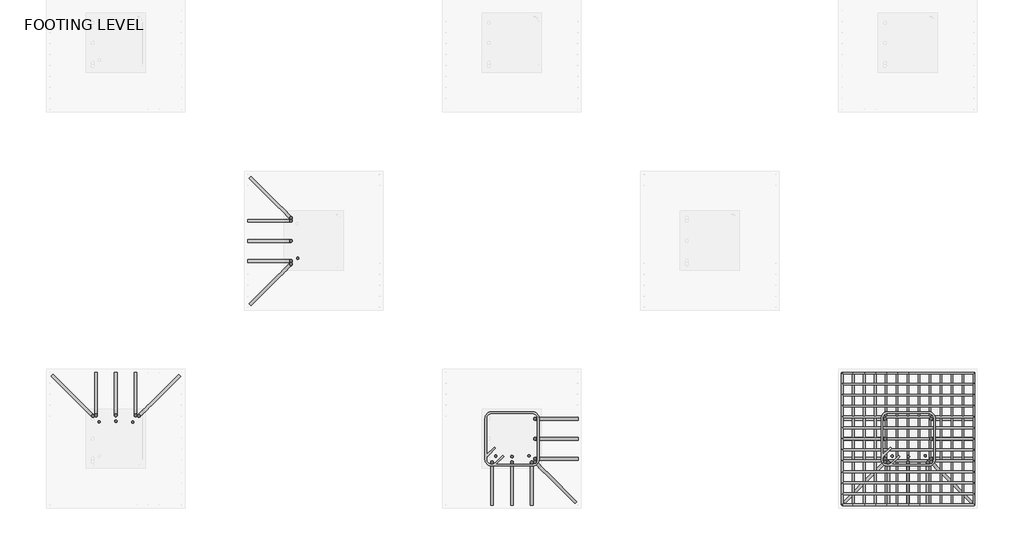
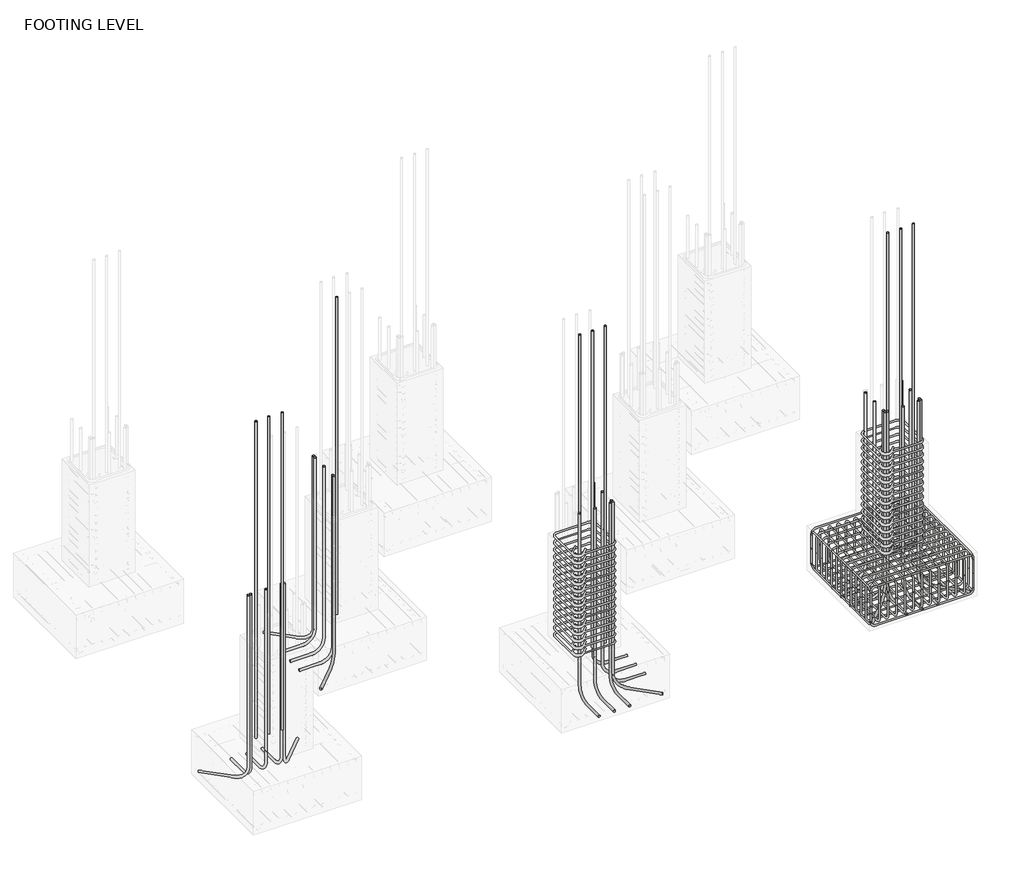
# One storey, part 3 of 10: 32 reinforcing bars.
"""IFC4 building model written with IfcOpenShell, lengths in millimetres."""

from ifc_helpers import new_model, si_unit, point, frame, origin, place, context, project, spatial, polyline, circle_curve, trimmed, segment, composite_curve, source, transform, mapped, element, save
from ifc_brep_helpers import swept_disk

model = new_model("IFC4")

# Units and contexts
model_context = context("Model", 3, world=origin())
ifc_project = project(units=[si_unit("LENGTHUNIT", "METRE", prefix="MILLI")], contexts=[model_context])

# Site, building, storey
site = spatial("IfcSite", under=ifc_project)
building = spatial("IfcBuilding", under=site)
storey = spatial("IfcBuildingStorey", under=building, Name="FOOTING LEVEL", Elevation=-2133.6)

# Reinforcing bars
placement = place(None, origin())
reinforcing_bar_shape = source(origin(), model_context, "Body", "SolidModel", [
    swept_disk(composite_curve([segment(polyline([(365.0730963, 756.4829396, -2583.0), (365.0730963, 756.4829396, -2905.1)]), True, "CONTINUOUS"), segment(trimmed(circle_curve(frame((274.8730963, 756.4829396, -2905.1), z_axis=(0.0, 1.0, 0.0), x_axis=(90.19999999999999, 0.0, 0.0)), 90.2), [point((365.0730963, 756.4829396, -2905.1))], [point((274.8730963, 756.4829396, -2995.3))], True, "CARTESIAN"), True, "CONTINUOUS"), segment(polyline([(274.8730963, 756.4829396, -2995.3), (-1572.9269037, 756.4829396, -2995.3)]), True, "CONTINUOUS"), segment(trimmed(circle_curve(frame((-1572.9269037, 756.4829396, -2905.1), z_axis=(0.0, 1.0, 0.0), x_axis=(0.0, 0.0, -90.20000000000027)), 90.2), [point((-1572.9269037, 756.4829396, -2995.3))], [point((-1663.1269037, 756.4829396, -2905.1))], True, "CARTESIAN"), True, "CONTINUOUS"), segment(polyline([(-1663.1269037, 756.4829396, -2905.1), (-1663.1269037, 756.4829396, -2583.0)]), True, "CONTINUOUS")], self_intersect=False), 12.7),
])
element("IfcReinforcingBar", 1, at=placement, inside=storey, context=model_context, shape_type="MappedRepresentation", body=[
    mapped(reinforcing_bar_shape, transform((0.0, 0.0, 0.0), x_axis=(1.0, 0.0, 0.0), y_axis=(0.0, 1.0, 0.0), z_axis=(0.0, 0.0, 1.0))),
    mapped(reinforcing_bar_shape, transform((0.0, -169.0166667, 0.0), x_axis=(1.0, 0.0, 0.0), y_axis=(0.0, 1.0, 0.0), z_axis=(0.0, 0.0, 1.0))),
    mapped(reinforcing_bar_shape, transform((0.0, -338.0333333, 0.0), x_axis=(1.0, 0.0, 0.0), y_axis=(0.0, 1.0, 0.0), z_axis=(0.0, 0.0, 1.0))),
    mapped(reinforcing_bar_shape, transform((0.0, -507.05, 0.0), x_axis=(1.0, 0.0, 0.0), y_axis=(0.0, 1.0, 0.0), z_axis=(0.0, 0.0, 1.0))),
    mapped(reinforcing_bar_shape, transform((0.0, -676.0666667, 0.0), x_axis=(1.0, 0.0, 0.0), y_axis=(0.0, 1.0, 0.0), z_axis=(0.0, 0.0, 1.0))),
    mapped(reinforcing_bar_shape, transform((0.0, -845.0833333, 0.0), x_axis=(1.0, 0.0, 0.0), y_axis=(0.0, 1.0, 0.0), z_axis=(0.0, 0.0, 1.0))),
    mapped(reinforcing_bar_shape, transform((0.0, -1014.1, 0.0), x_axis=(1.0, 0.0, 0.0), y_axis=(0.0, 1.0, 0.0), z_axis=(0.0, 0.0, 1.0))),
    mapped(reinforcing_bar_shape, transform((0.0, -1183.1166667, 0.0), x_axis=(1.0, 0.0, 0.0), y_axis=(0.0, 1.0, 0.0), z_axis=(0.0, 0.0, 1.0))),
    mapped(reinforcing_bar_shape, transform((0.0, -1352.1333333, 0.0), x_axis=(1.0, 0.0, 0.0), y_axis=(0.0, 1.0, 0.0), z_axis=(0.0, 0.0, 1.0))),
    mapped(reinforcing_bar_shape, transform((0.0, -1521.15, 0.0), x_axis=(1.0, 0.0, 0.0), y_axis=(0.0, 1.0, 0.0), z_axis=(0.0, 0.0, 1.0))),
    mapped(reinforcing_bar_shape, transform((0.0, -1690.1666667, 0.0), x_axis=(1.0, 0.0, 0.0), y_axis=(0.0, 1.0, 0.0), z_axis=(0.0, 0.0, 1.0))),
    mapped(reinforcing_bar_shape, transform((0.0, -1859.1833333, 0.0), x_axis=(1.0, 0.0, 0.0), y_axis=(0.0, 1.0, 0.0), z_axis=(0.0, 0.0, 1.0))),
    mapped(reinforcing_bar_shape, transform((0.0, -2028.2, 0.0), x_axis=(1.0, 0.0, 0.0), y_axis=(0.0, 1.0, 0.0), z_axis=(0.0, 0.0, 1.0))),
])
reinforcing_bar_2_shape = source(origin(), model_context, "Body", "SolidModel", [
    swept_disk(composite_curve([segment(polyline([(-1663.1269037, 756.4829396, -2598.6), (-1663.1269037, 756.4829396, -2276.5)]), True, "CONTINUOUS"), segment(trimmed(circle_curve(frame((-1572.9269037, 756.4829396, -2276.5), z_axis=(0.0, 1.0, 0.0), x_axis=(-90.20000000000005, 0.0, 0.0)), 90.2), [point((-1663.1269037, 756.4829396, -2276.5))], [point((-1572.9269037, 756.4829396, -2186.3))], True, "CARTESIAN"), True, "CONTINUOUS"), segment(polyline([(-1572.9269037, 756.4829396, -2186.3), (274.8730963, 756.4829396, -2186.3)]), True, "CONTINUOUS"), segment(trimmed(circle_curve(frame((274.8730963, 756.4829396, -2276.5), z_axis=(0.0, 1.0, 0.0), x_axis=(0.0, 0.0, 90.19999999999982)), 90.2), [point((274.8730963, 756.4829396, -2186.3))], [point((365.0730963, 756.4829396, -2276.5))], True, "CARTESIAN"), True, "CONTINUOUS"), segment(polyline([(365.0730963, 756.4829396, -2276.5), (365.0730963, 756.4829396, -2598.6)]), True, "CONTINUOUS")], self_intersect=False), 12.7),
])
element("IfcReinforcingBar", 2, at=placement, inside=storey, context=model_context, shape_type="MappedRepresentation", body=[
    mapped(reinforcing_bar_2_shape, transform((0.0, 0.0, 0.0), x_axis=(1.0, 0.0, 0.0), y_axis=(0.0, 1.0, 0.0), z_axis=(0.0, 0.0, 1.0))),
    mapped(reinforcing_bar_2_shape, transform((0.0, -169.0166667, 0.0), x_axis=(1.0, 0.0, 0.0), y_axis=(0.0, 1.0, 0.0), z_axis=(0.0, 0.0, 1.0))),
    mapped(reinforcing_bar_2_shape, transform((0.0, -338.0333333, 0.0), x_axis=(1.0, 0.0, 0.0), y_axis=(0.0, 1.0, 0.0), z_axis=(0.0, 0.0, 1.0))),
    mapped(reinforcing_bar_2_shape, transform((0.0, -507.05, 0.0), x_axis=(1.0, 0.0, 0.0), y_axis=(0.0, 1.0, 0.0), z_axis=(0.0, 0.0, 1.0))),
    mapped(reinforcing_bar_2_shape, transform((0.0, -676.0666667, 0.0), x_axis=(1.0, 0.0, 0.0), y_axis=(0.0, 1.0, 0.0), z_axis=(0.0, 0.0, 1.0))),
    mapped(reinforcing_bar_2_shape, transform((0.0, -845.0833333, 0.0), x_axis=(1.0, 0.0, 0.0), y_axis=(0.0, 1.0, 0.0), z_axis=(0.0, 0.0, 1.0))),
    mapped(reinforcing_bar_2_shape, transform((0.0, -1014.1, 0.0), x_axis=(1.0, 0.0, 0.0), y_axis=(0.0, 1.0, 0.0), z_axis=(0.0, 0.0, 1.0))),
    mapped(reinforcing_bar_2_shape, transform((0.0, -1183.1166667, 0.0), x_axis=(1.0, 0.0, 0.0), y_axis=(0.0, 1.0, 0.0), z_axis=(0.0, 0.0, 1.0))),
    mapped(reinforcing_bar_2_shape, transform((0.0, -1352.1333333, 0.0), x_axis=(1.0, 0.0, 0.0), y_axis=(0.0, 1.0, 0.0), z_axis=(0.0, 0.0, 1.0))),
    mapped(reinforcing_bar_2_shape, transform((0.0, -1521.15, 0.0), x_axis=(1.0, 0.0, 0.0), y_axis=(0.0, 1.0, 0.0), z_axis=(0.0, 0.0, 1.0))),
    mapped(reinforcing_bar_2_shape, transform((0.0, -1690.1666667, 0.0), x_axis=(1.0, 0.0, 0.0), y_axis=(0.0, 1.0, 0.0), z_axis=(0.0, 0.0, 1.0))),
    mapped(reinforcing_bar_2_shape, transform((0.0, -1859.1833333, 0.0), x_axis=(1.0, 0.0, 0.0), y_axis=(0.0, 1.0, 0.0), z_axis=(0.0, 0.0, 1.0))),
    mapped(reinforcing_bar_2_shape, transform((0.0, -2028.2, 0.0), x_axis=(1.0, 0.0, 0.0), y_axis=(0.0, 1.0, 0.0), z_axis=(0.0, 0.0, 1.0))),
])
reinforcing_bar_3_shape = source(origin(), model_context, "Body", "SolidModel", [
    swept_disk(composite_curve([segment(polyline([(365.0730963, -1271.7170604, -2559.4978077), (365.0730963, -1271.7170604, -2881.5978077)]), True, "CONTINUOUS"), segment(trimmed(circle_curve(frame((365.0730963, -1181.5170604, -2881.5978077), z_axis=(1.0, 0.0, 0.0), x_axis=(0.0, -90.20000000000005, 0.0)), 90.2), [point((365.0730963, -1271.7170604, -2881.5978077))], [point((365.0730963, -1181.5170604, -2971.7978077))], True, "CARTESIAN"), True, "CONTINUOUS"), segment(polyline([(365.0730963, -1181.5170604, -2971.7978077), (365.0730963, 666.2829396, -2971.7978077)]), True, "CONTINUOUS"), segment(trimmed(circle_curve(frame((365.0730963, 666.2829396, -2881.5978077), z_axis=(1.0, 0.0, 0.0), x_axis=(0.0, 0.0, -90.19999999999982)), 90.2), [point((365.0730963, 666.2829396, -2971.7978077))], [point((365.0730963, 756.4829396, -2881.5978077))], True, "CARTESIAN"), True, "CONTINUOUS"), segment(polyline([(365.0730963, 756.4829396, -2881.5978077), (365.0730963, 756.4829396, -2559.4978077)]), True, "CONTINUOUS")], self_intersect=False), 12.7),
])
element("IfcReinforcingBar", 3, at=placement, inside=storey, context=model_context, shape_type="MappedRepresentation", body=[
    mapped(reinforcing_bar_3_shape, transform((0.0, 0.0, 0.0), x_axis=(1.0, 0.0, 0.0), y_axis=(0.0, 1.0, 0.0), z_axis=(0.0, 0.0, 1.0))),
    mapped(reinforcing_bar_3_shape, transform((-169.0166667, 0.0, 0.0), x_axis=(1.0, 0.0, 0.0), y_axis=(0.0, 1.0, 0.0), z_axis=(0.0, 0.0, 1.0))),
    mapped(reinforcing_bar_3_shape, transform((-338.0333333, 0.0, 0.0), x_axis=(1.0, 0.0, 0.0), y_axis=(0.0, 1.0, 0.0), z_axis=(0.0, 0.0, 1.0))),
    mapped(reinforcing_bar_3_shape, transform((-507.05, 0.0, 0.0), x_axis=(1.0, 0.0, 0.0), y_axis=(0.0, 1.0, 0.0), z_axis=(0.0, 0.0, 1.0))),
    mapped(reinforcing_bar_3_shape, transform((-676.0666667, 0.0, 0.0), x_axis=(1.0, 0.0, 0.0), y_axis=(0.0, 1.0, 0.0), z_axis=(0.0, 0.0, 1.0))),
    mapped(reinforcing_bar_3_shape, transform((-845.0833333, 0.0, 0.0), x_axis=(1.0, 0.0, 0.0), y_axis=(0.0, 1.0, 0.0), z_axis=(0.0, 0.0, 1.0))),
    mapped(reinforcing_bar_3_shape, transform((-1014.1, 0.0, 0.0), x_axis=(1.0, 0.0, 0.0), y_axis=(0.0, 1.0, 0.0), z_axis=(0.0, 0.0, 1.0))),
    mapped(reinforcing_bar_3_shape, transform((-1183.1166667, 0.0, 0.0), x_axis=(1.0, 0.0, 0.0), y_axis=(0.0, 1.0, 0.0), z_axis=(0.0, 0.0, 1.0))),
    mapped(reinforcing_bar_3_shape, transform((-1352.1333333, 0.0, 0.0), x_axis=(1.0, 0.0, 0.0), y_axis=(0.0, 1.0, 0.0), z_axis=(0.0, 0.0, 1.0))),
    mapped(reinforcing_bar_3_shape, transform((-1521.15, 0.0, 0.0), x_axis=(1.0, 0.0, 0.0), y_axis=(0.0, 1.0, 0.0), z_axis=(0.0, 0.0, 1.0))),
    mapped(reinforcing_bar_3_shape, transform((-1690.1666667, 0.0, 0.0), x_axis=(1.0, 0.0, 0.0), y_axis=(0.0, 1.0, 0.0), z_axis=(0.0, 0.0, 1.0))),
    mapped(reinforcing_bar_3_shape, transform((-1859.1833333, 0.0, 0.0), x_axis=(1.0, 0.0, 0.0), y_axis=(0.0, 1.0, 0.0), z_axis=(0.0, 0.0, 1.0))),
    mapped(reinforcing_bar_3_shape, transform((-2028.2, 0.0, 0.0), x_axis=(1.0, 0.0, 0.0), y_axis=(0.0, 1.0, 0.0), z_axis=(0.0, 0.0, 1.0))),
])
reinforcing_bar_4_shape = source(origin(), model_context, "Body", "SolidModel", [
    swept_disk(composite_curve([segment(polyline([(-1663.1269037, -1271.7170604, -2622.9919875), (-1663.1269037, -1271.7170604, -2300.8919875)]), True, "CONTINUOUS"), segment(trimmed(circle_curve(frame((-1663.1269037, -1181.5170604, -2300.8919875), z_axis=(-1.0, 0.0, 0.0), x_axis=(0.0, -90.20000000000005, 0.0)), 90.2), [point((-1663.1269037, -1271.7170604, -2300.8919875))], [point((-1663.1269037, -1181.5170604, -2210.6919875))], True, "CARTESIAN"), True, "CONTINUOUS"), segment(polyline([(-1663.1269037, -1181.5170604, -2210.6919875), (-1663.1269037, 666.2829396, -2210.6919875)]), True, "CONTINUOUS"), segment(trimmed(circle_curve(frame((-1663.1269037, 666.2829396, -2300.8919875), z_axis=(-1.0, 0.0, 0.0), x_axis=(0.0, 0.0, 90.20000000000027)), 90.2), [point((-1663.1269037, 666.2829396, -2210.6919875))], [point((-1663.1269037, 756.4829396, -2300.8919875))], True, "CARTESIAN"), True, "CONTINUOUS"), segment(polyline([(-1663.1269037, 756.4829396, -2300.8919875), (-1663.1269037, 756.4829396, -2622.9919875)]), True, "CONTINUOUS")], self_intersect=False), 12.7),
])
element("IfcReinforcingBar", 4, at=placement, inside=storey, context=model_context, shape_type="MappedRepresentation", body=[
    mapped(reinforcing_bar_4_shape, transform((0.0, 0.0, 0.0), x_axis=(1.0, 0.0, 0.0), y_axis=(0.0, 1.0, 0.0), z_axis=(0.0, 0.0, 1.0))),
    mapped(reinforcing_bar_4_shape, transform((169.0166667, 0.0, 0.0), x_axis=(1.0, 0.0, 0.0), y_axis=(0.0, 1.0, 0.0), z_axis=(0.0, 0.0, 1.0))),
    mapped(reinforcing_bar_4_shape, transform((338.0333333, 0.0, 0.0), x_axis=(1.0, 0.0, 0.0), y_axis=(0.0, 1.0, 0.0), z_axis=(0.0, 0.0, 1.0))),
    mapped(reinforcing_bar_4_shape, transform((507.05, 0.0, 0.0), x_axis=(1.0, 0.0, 0.0), y_axis=(0.0, 1.0, 0.0), z_axis=(0.0, 0.0, 1.0))),
    mapped(reinforcing_bar_4_shape, transform((676.0666667, 0.0, 0.0), x_axis=(1.0, 0.0, 0.0), y_axis=(0.0, 1.0, 0.0), z_axis=(0.0, 0.0, 1.0))),
    mapped(reinforcing_bar_4_shape, transform((845.0833333, 0.0, 0.0), x_axis=(1.0, 0.0, 0.0), y_axis=(0.0, 1.0, 0.0), z_axis=(0.0, 0.0, 1.0))),
    mapped(reinforcing_bar_4_shape, transform((1014.1, 0.0, 0.0), x_axis=(1.0, 0.0, 0.0), y_axis=(0.0, 1.0, 0.0), z_axis=(0.0, 0.0, 1.0))),
    mapped(reinforcing_bar_4_shape, transform((1183.1166667, 0.0, 0.0), x_axis=(1.0, 0.0, 0.0), y_axis=(0.0, 1.0, 0.0), z_axis=(0.0, 0.0, 1.0))),
    mapped(reinforcing_bar_4_shape, transform((1352.1333333, 0.0, 0.0), x_axis=(1.0, 0.0, 0.0), y_axis=(0.0, 1.0, 0.0), z_axis=(0.0, 0.0, 1.0))),
    mapped(reinforcing_bar_4_shape, transform((1521.15, 0.0, 0.0), x_axis=(1.0, 0.0, 0.0), y_axis=(0.0, 1.0, 0.0), z_axis=(0.0, 0.0, 1.0))),
    mapped(reinforcing_bar_4_shape, transform((1690.1666667, 0.0, 0.0), x_axis=(1.0, 0.0, 0.0), y_axis=(0.0, 1.0, 0.0), z_axis=(0.0, 0.0, 1.0))),
    mapped(reinforcing_bar_4_shape, transform((1859.1833333, 0.0, 0.0), x_axis=(1.0, 0.0, 0.0), y_axis=(0.0, 1.0, 0.0), z_axis=(0.0, 0.0, 1.0))),
    mapped(reinforcing_bar_4_shape, transform((2028.2, 0.0, 0.0), x_axis=(1.0, 0.0, 0.0), y_axis=(0.0, 1.0, 0.0), z_axis=(0.0, 0.0, 1.0))),
])
reinforcing_bar_5_shape = source(origin(), model_context, "Body", "SolidModel", [
    swept_disk(composite_curve([segment(polyline([(-6882.1462687, -522.2984887, 0.0), (-6995.545872, -635.6980921, 0.0)]), True, "CONTINUOUS"), segment(trimmed(circle_curve(frame((-7059.3269037, -571.9170604, 0.0), z_axis=(0.0, 0.0, -1.0), x_axis=(63.78103170000031, -63.781031700000085, 0.0)), 90.2), [point((-6995.545872, -635.6980921, 0.0))], [point((-7149.5269037, -571.9170604, 0.0))], True, "CARTESIAN"), True, "CONTINUOUS"), segment(polyline([(-7149.5269037, -571.9170604, 0.0), (-7149.5269037, 56.6829396, 0.0)]), True, "CONTINUOUS"), segment(trimmed(circle_curve(frame((-7059.3269037, 56.6829396, 0.0), z_axis=(0.0, 0.0, -1.0), x_axis=(-90.19999999999982, 0.0, 0.0)), 90.2), [point((-7149.5269037, 56.6829396, 0.0))], [point((-7059.3269037, 146.8829396, 0.0))], True, "CARTESIAN"), True, "CONTINUOUS"), segment(polyline([(-7059.3269037, 146.8829396, 0.0), (-6430.7269037, 146.8829396, 0.0)]), True, "CONTINUOUS"), segment(trimmed(circle_curve(frame((-6430.7269037, 56.7273645, 2.8305953), z_axis=(0.0, -0.03138132276777647, -0.9995074850051623), x_axis=(0.0, 90.1555751, -2.8305953)), 90.2), [point((-6430.7269037, 146.8829396, 0.0))], [point((-6340.5269037, 56.7273645, 2.8305953))], True, "CARTESIAN"), True, "CONTINUOUS"), segment(polyline([(-6340.5269037, 56.7273645, 2.8305953), (-6340.5269037, -571.9614853, 22.5694047)]), True, "CONTINUOUS"), segment(trimmed(circle_curve(frame((-6430.7269037, -571.9614853, 22.5694047), z_axis=(0.0, -0.03138132276777647, -0.9995074850051623), x_axis=(90.19999999999982, 0.0, 0.0)), 90.2), [point((-6340.5269037, -571.9614853, 22.5694047))], [point((-6430.7269037, -662.1170604, 25.4))], True, "CARTESIAN"), True, "CONTINUOUS"), segment(polyline([(-6430.7269037, -662.1170604, 25.4), (-7059.3269037, -662.1170604, 25.4)]), True, "CONTINUOUS"), segment(trimmed(circle_curve(frame((-7059.3269037, -571.9170604, 25.4), z_axis=(0.0, 0.0, -1.0), x_axis=(0.0, -90.20000000000005, 0.0)), 90.2), [point((-7059.3269037, -662.1170604, 25.4))], [point((-7123.1079353, -508.1360287, 25.4))], True, "CARTESIAN"), True, "CONTINUOUS"), segment(polyline([(-7123.1079353, -508.1360287, 25.4), (-7009.708332, -394.7364254, 25.4)]), True, "CONTINUOUS")], self_intersect=False), 12.7),
])
element("IfcReinforcingBar", 5, at=placement, inside=storey, context=model_context, shape_type="MappedRepresentation", body=[
    mapped(reinforcing_bar_5_shape, transform((0.0, 0.0, 0.0), x_axis=(1.0, 0.0, 0.0), y_axis=(0.0, 1.0, 0.0), z_axis=(0.0, 0.0, 1.0))),
    mapped(reinforcing_bar_5_shape, transform((0.0, 0.0, -148.6357143), x_axis=(1.0, 0.0, 0.0), y_axis=(0.0, 1.0, 0.0), z_axis=(0.0, 0.0, 1.0))),
    mapped(reinforcing_bar_5_shape, transform((0.0, 0.0, -297.2714286), x_axis=(1.0, 0.0, 0.0), y_axis=(0.0, 1.0, 0.0), z_axis=(0.0, 0.0, 1.0))),
    mapped(reinforcing_bar_5_shape, transform((0.0, 0.0, -445.9071429), x_axis=(1.0, 0.0, 0.0), y_axis=(0.0, 1.0, 0.0), z_axis=(0.0, 0.0, 1.0))),
    mapped(reinforcing_bar_5_shape, transform((0.0, 0.0, -594.5428571), x_axis=(1.0, 0.0, 0.0), y_axis=(0.0, 1.0, 0.0), z_axis=(0.0, 0.0, 1.0))),
    mapped(reinforcing_bar_5_shape, transform((0.0, 0.0, -743.1785714), x_axis=(1.0, 0.0, 0.0), y_axis=(0.0, 1.0, 0.0), z_axis=(0.0, 0.0, 1.0))),
    mapped(reinforcing_bar_5_shape, transform((0.0, 0.0, -891.8142857), x_axis=(1.0, 0.0, 0.0), y_axis=(0.0, 1.0, 0.0), z_axis=(0.0, 0.0, 1.0))),
    mapped(reinforcing_bar_5_shape, transform((0.0, 0.0, -1040.45), x_axis=(1.0, 0.0, 0.0), y_axis=(0.0, 1.0, 0.0), z_axis=(0.0, 0.0, 1.0))),
    mapped(reinforcing_bar_5_shape, transform((0.0, 0.0, -1189.0857143), x_axis=(1.0, 0.0, 0.0), y_axis=(0.0, 1.0, 0.0), z_axis=(0.0, 0.0, 1.0))),
    mapped(reinforcing_bar_5_shape, transform((0.0, 0.0, -1337.7214286), x_axis=(1.0, 0.0, 0.0), y_axis=(0.0, 1.0, 0.0), z_axis=(0.0, 0.0, 1.0))),
    mapped(reinforcing_bar_5_shape, transform((0.0, 0.0, -1486.3571429), x_axis=(1.0, 0.0, 0.0), y_axis=(0.0, 1.0, 0.0), z_axis=(0.0, 0.0, 1.0))),
    mapped(reinforcing_bar_5_shape, transform((0.0, 0.0, -1634.9928571), x_axis=(1.0, 0.0, 0.0), y_axis=(0.0, 1.0, 0.0), z_axis=(0.0, 0.0, 1.0))),
    mapped(reinforcing_bar_5_shape, transform((0.0, 0.0, -1783.6285714), x_axis=(1.0, 0.0, 0.0), y_axis=(0.0, 1.0, 0.0), z_axis=(0.0, 0.0, 1.0))),
    mapped(reinforcing_bar_5_shape, transform((0.0, 0.0, -1932.2642857), x_axis=(1.0, 0.0, 0.0), y_axis=(0.0, 1.0, 0.0), z_axis=(0.0, 0.0, 1.0))),
    mapped(reinforcing_bar_5_shape, transform((0.0, 0.0, -2080.9), x_axis=(1.0, 0.0, 0.0), y_axis=(0.0, 1.0, 0.0), z_axis=(0.0, 0.0, 1.0))),
])
reinforcing_bar_6_shape = source(origin(), model_context, "Body", "SolidModel", [
    swept_disk(composite_curve([segment(polyline([(-786.1462687, -522.2984887, 0.0), (-899.545872, -635.6980921, 0.0)]), True, "CONTINUOUS"), segment(trimmed(circle_curve(frame((-963.3269037, -571.9170604, 0.0), z_axis=(0.0, 0.0, -1.0), x_axis=(63.78103169999997, -63.781031700000085, 0.0)), 90.2), [point((-899.545872, -635.6980921, 0.0))], [point((-1053.5269037, -571.9170604, 0.0))], True, "CARTESIAN"), True, "CONTINUOUS"), segment(polyline([(-1053.5269037, -571.9170604, 0.0), (-1053.5269037, 56.6829396, 0.0)]), True, "CONTINUOUS"), segment(trimmed(circle_curve(frame((-963.3269037, 56.6829396, 0.0), z_axis=(0.0, 0.0, -1.0), x_axis=(-90.20000000000005, 0.0, 0.0)), 90.2), [point((-1053.5269037, 56.6829396, 0.0))], [point((-963.3269037, 146.8829396, 0.0))], True, "CARTESIAN"), True, "CONTINUOUS"), segment(polyline([(-963.3269037, 146.8829396, 0.0), (-334.7269037, 146.8829396, 0.0)]), True, "CONTINUOUS"), segment(trimmed(circle_curve(frame((-334.7269037, 56.7273645, 2.8305953), z_axis=(0.0, -0.03138132276777647, -0.9995074850051623), x_axis=(0.0, 90.1555751, -2.8305953)), 90.2), [point((-334.7269037, 146.8829396, 0.0))], [point((-244.5269037, 56.7273645, 2.8305953))], True, "CARTESIAN"), True, "CONTINUOUS"), segment(polyline([(-244.5269037, 56.7273645, 2.8305953), (-244.5269037, -571.9614853, 22.5694047)]), True, "CONTINUOUS"), segment(trimmed(circle_curve(frame((-334.7269037, -571.9614853, 22.5694047), z_axis=(0.0, -0.03138132276777647, -0.9995074850051623), x_axis=(90.19999999999999, 0.0, 0.0)), 90.2), [point((-244.5269037, -571.9614853, 22.5694047))], [point((-334.7269037, -662.1170604, 25.4))], True, "CARTESIAN"), True, "CONTINUOUS"), segment(polyline([(-334.7269037, -662.1170604, 25.4), (-963.3269037, -662.1170604, 25.4)]), True, "CONTINUOUS"), segment(trimmed(circle_curve(frame((-963.3269037, -571.9170604, 25.4), z_axis=(0.0, 0.0, -1.0), x_axis=(0.0, -90.20000000000005, 0.0)), 90.2), [point((-963.3269037, -662.1170604, 25.4))], [point((-1027.1079353, -508.1360287, 25.4))], True, "CARTESIAN"), True, "CONTINUOUS"), segment(polyline([(-1027.1079353, -508.1360287, 25.4), (-913.708332, -394.7364254, 25.4)]), True, "CONTINUOUS")], self_intersect=False), 12.7),
])
element("IfcReinforcingBar", 6, at=placement, inside=storey, context=model_context, shape_type="MappedRepresentation", body=[
    mapped(reinforcing_bar_6_shape, transform((0.0, 0.0, 0.0), x_axis=(1.0, 0.0, 0.0), y_axis=(0.0, 1.0, 0.0), z_axis=(0.0, 0.0, 1.0))),
    mapped(reinforcing_bar_6_shape, transform((0.0, 0.0, -148.6357143), x_axis=(1.0, 0.0, 0.0), y_axis=(0.0, 1.0, 0.0), z_axis=(0.0, 0.0, 1.0))),
    mapped(reinforcing_bar_6_shape, transform((0.0, 0.0, -297.2714286), x_axis=(1.0, 0.0, 0.0), y_axis=(0.0, 1.0, 0.0), z_axis=(0.0, 0.0, 1.0))),
    mapped(reinforcing_bar_6_shape, transform((0.0, 0.0, -445.9071429), x_axis=(1.0, 0.0, 0.0), y_axis=(0.0, 1.0, 0.0), z_axis=(0.0, 0.0, 1.0))),
    mapped(reinforcing_bar_6_shape, transform((0.0, 0.0, -594.5428571), x_axis=(1.0, 0.0, 0.0), y_axis=(0.0, 1.0, 0.0), z_axis=(0.0, 0.0, 1.0))),
    mapped(reinforcing_bar_6_shape, transform((0.0, 0.0, -743.1785714), x_axis=(1.0, 0.0, 0.0), y_axis=(0.0, 1.0, 0.0), z_axis=(0.0, 0.0, 1.0))),
    mapped(reinforcing_bar_6_shape, transform((0.0, 0.0, -891.8142857), x_axis=(1.0, 0.0, 0.0), y_axis=(0.0, 1.0, 0.0), z_axis=(0.0, 0.0, 1.0))),
    mapped(reinforcing_bar_6_shape, transform((0.0, 0.0, -1040.45), x_axis=(1.0, 0.0, 0.0), y_axis=(0.0, 1.0, 0.0), z_axis=(0.0, 0.0, 1.0))),
    mapped(reinforcing_bar_6_shape, transform((0.0, 0.0, -1189.0857143), x_axis=(1.0, 0.0, 0.0), y_axis=(0.0, 1.0, 0.0), z_axis=(0.0, 0.0, 1.0))),
    mapped(reinforcing_bar_6_shape, transform((0.0, 0.0, -1337.7214286), x_axis=(1.0, 0.0, 0.0), y_axis=(0.0, 1.0, 0.0), z_axis=(0.0, 0.0, 1.0))),
    mapped(reinforcing_bar_6_shape, transform((0.0, 0.0, -1486.3571429), x_axis=(1.0, 0.0, 0.0), y_axis=(0.0, 1.0, 0.0), z_axis=(0.0, 0.0, 1.0))),
    mapped(reinforcing_bar_6_shape, transform((0.0, 0.0, -1634.9928571), x_axis=(1.0, 0.0, 0.0), y_axis=(0.0, 1.0, 0.0), z_axis=(0.0, 0.0, 1.0))),
    mapped(reinforcing_bar_6_shape, transform((0.0, 0.0, -1783.6285714), x_axis=(1.0, 0.0, 0.0), y_axis=(0.0, 1.0, 0.0), z_axis=(0.0, 0.0, 1.0))),
    mapped(reinforcing_bar_6_shape, transform((0.0, 0.0, -1932.2642857), x_axis=(1.0, 0.0, 0.0), y_axis=(0.0, 1.0, 0.0), z_axis=(0.0, 0.0, 1.0))),
    mapped(reinforcing_bar_6_shape, transform((0.0, 0.0, -2080.9), x_axis=(1.0, 0.0, 0.0), y_axis=(0.0, 1.0, 0.0), z_axis=(0.0, 0.0, 1.0))),
])
element("IfcReinforcingBar", 7, at=placement, inside=storey, context=model_context, shape_type="SolidModel", body=[
    swept_disk(composite_curve([segment(polyline([(331.4269893, -1238.0709533, -2976.5), (-115.5238015, -791.1201626, -2976.5)]), True, "CONTINUOUS"), segment(trimmed(circle_curve(frame((-115.5238015, -791.1201626, -2722.5), z_axis=(0.7071067811865508, 0.7071067811865444, 0.0), x_axis=(0.0, 0.0, -254.0)), 254.0), [point((-115.5238015, -791.1201626, -2976.5))], [point((-295.1289239, -611.5150401, -2722.5))], True, "CARTESIAN"), True, "CONTINUOUS"), segment(polyline([(-295.1289239, -611.5150401, -2722.5), (-295.1289239, -611.5150401, 874.4)]), True, "CONTINUOUS")], self_intersect=False), 21.5),
])
element("IfcReinforcingBar", 8, at=placement, inside=storey, context=model_context, shape_type="SolidModel", body=[
    swept_disk(composite_curve([segment(polyline([(-1629.4807966, -1238.0709533, -2976.5), (-1182.5300058, -791.1201626, -2976.5)]), True, "CONTINUOUS"), segment(trimmed(circle_curve(frame((-1182.5300058, -791.1201626, -2722.5), z_axis=(0.7071067811865475, -0.7071067811865477, 0.0), x_axis=(0.0, 0.0, -254.0)), 254.0), [point((-1182.5300058, -791.1201626, -2976.5))], [point((-1002.9248834, -611.5150401, -2722.5))], True, "CARTESIAN"), True, "CONTINUOUS"), segment(polyline([(-1002.9248834, -611.5150401, -2722.5), (-1002.9248834, -611.5150401, 874.4)]), True, "CONTINUOUS")], self_intersect=False), 21.5),
])
element("IfcReinforcingBar", 9, at=placement, inside=storey, context=model_context, shape_type="SolidModel", body=[
    swept_disk(composite_curve([segment(polyline([(331.4269893, -1238.0709533, -2976.5), (-115.5238015, -791.1201626, -2976.5)]), True, "CONTINUOUS"), segment(trimmed(circle_curve(frame((-115.5238015, -791.1201626, -2722.5), z_axis=(0.7071067811865508, 0.7071067811865444, 0.0), x_axis=(0.0, 0.0, -254.0)), 254.0), [point((-115.5238015, -791.1201626, -2976.5))], [point((-295.1289239, -611.5150401, -2722.5))], True, "CARTESIAN"), True, "CONTINUOUS"), segment(polyline([(-295.1289239, -611.5150401, -2722.5), (-295.1289239, -611.5150401, 874.4)]), True, "CONTINUOUS")], self_intersect=False), 21.5),
])
reinforcing_bar_7_shape = source(origin(), model_context, "Body", "SolidModel", [
    swept_disk(composite_curve([segment(polyline([(367.7730963, -565.9980034, -2976.5), (-41.1289239, -565.9980034, -2976.5)]), True, "CONTINUOUS"), segment(trimmed(circle_curve(frame((-41.1289239, -565.9980034, -2722.5), z_axis=(0.0, 1.0, 0.0), x_axis=(0.0, 0.0, -254.0)), 254.0), [point((-41.1289239, -565.9980034, -2976.5))], [point((-295.1289239, -565.9980034, -2722.5))], True, "CARTESIAN"), True, "CONTINUOUS"), segment(polyline([(-295.1289239, -565.9980034, -2722.5), (-295.1289239, -565.9980034, 874.4)]), True, "CONTINUOUS")], self_intersect=False), 21.5),
])
element("IfcReinforcingBar", 10, at=placement, inside=storey, context=model_context, shape_type="MappedRepresentation", body=[
    mapped(reinforcing_bar_7_shape, transform((0.0, 0.0, 0.0), x_axis=(1.0, 0.0, 0.0), y_axis=(0.0, 1.0, 0.0), z_axis=(0.0, 0.0, 1.0))),
    mapped(reinforcing_bar_7_shape, transform((0.0, 309.128507, 0.0), x_axis=(1.0, 0.0, 0.0), y_axis=(0.0, 1.0, 0.0), z_axis=(0.0, 0.0, 1.0))),
    mapped(reinforcing_bar_7_shape, transform((0.0, 618.2570139, 0.0), x_axis=(1.0, 0.0, 0.0), y_axis=(0.0, 1.0, 0.0), z_axis=(0.0, 0.0, 1.0))),
])
reinforcing_bar_8_shape = source(origin(), model_context, "Body", "SolidModel", [
    swept_disk(composite_curve([segment(polyline([(-1665.8269037, -565.9980034, -2976.5), (-1256.9248834, -565.9980034, -2976.5)]), True, "CONTINUOUS"), segment(trimmed(circle_curve(frame((-1256.9248834, -565.9980034, -2722.5), z_axis=(0.0, -1.0, 0.0), x_axis=(0.0, 0.0, -254.0)), 254.0), [point((-1256.9248834, -565.9980034, -2976.5))], [point((-1002.9248834, -565.9980034, -2722.5))], True, "CARTESIAN"), True, "CONTINUOUS"), segment(polyline([(-1002.9248834, -565.9980034, -2722.5), (-1002.9248834, -565.9980034, 874.4)]), True, "CONTINUOUS")], self_intersect=False), 21.5),
])
element("IfcReinforcingBar", 11, at=placement, inside=storey, context=model_context, shape_type="MappedRepresentation", body=[
    mapped(reinforcing_bar_8_shape, transform((0.0, 0.0, 0.0), x_axis=(1.0, 0.0, 0.0), y_axis=(0.0, 1.0, 0.0), z_axis=(0.0, 0.0, 1.0))),
    mapped(reinforcing_bar_8_shape, transform((0.0, 309.128507, 0.0), x_axis=(1.0, 0.0, 0.0), y_axis=(0.0, 1.0, 0.0), z_axis=(0.0, 0.0, 1.0))),
    mapped(reinforcing_bar_8_shape, transform((0.0, 618.2570139, 0.0), x_axis=(1.0, 0.0, 0.0), y_axis=(0.0, 1.0, 0.0), z_axis=(0.0, 0.0, 1.0))),
])
reinforcing_bar_9_shape = source(origin(), model_context, "Body", "SolidModel", [
    swept_disk(composite_curve([segment(polyline([(-345.6587573, -1282.6598713, -2976.5), (-345.6587573, -873.757851, -2976.5)]), True, "CONTINUOUS"), segment(trimmed(circle_curve(frame((-345.6587573, -873.757851, -2722.5), z_axis=(1.0, 0.0, 0.0), x_axis=(0.0, 0.0, -254.0)), 254.0), [point((-345.6587573, -873.757851, -2976.5))], [point((-345.6587573, -619.757851, -2722.5))], True, "CARTESIAN"), True, "CONTINUOUS"), segment(polyline([(-345.6587573, -619.757851, -2722.5), (-345.6587573, -619.757851, 874.4)]), True, "CONTINUOUS")], self_intersect=False), 21.5),
])
element("IfcReinforcingBar", 12, at=placement, inside=storey, context=model_context, shape_type="MappedRepresentation", body=[
    mapped(reinforcing_bar_9_shape, transform((0.0, 0.0, 0.0), x_axis=(1.0, 0.0, 0.0), y_axis=(0.0, 1.0, 0.0), z_axis=(0.0, 0.0, 1.0))),
    mapped(reinforcing_bar_9_shape, transform((-304.9765997, 0.0, 0.0), x_axis=(1.0, 0.0, 0.0), y_axis=(0.0, 1.0, 0.0), z_axis=(0.0, 0.0, 1.0))),
    mapped(reinforcing_bar_9_shape, transform((-609.9531995, 0.0, 0.0), x_axis=(1.0, 0.0, 0.0), y_axis=(0.0, 1.0, 0.0), z_axis=(0.0, 0.0, 1.0))),
])
element("IfcReinforcingBar", 13, at=placement, inside=storey, context=model_context, shape_type="SolidModel", body=[
    swept_disk(composite_curve([segment(polyline([(-5764.5730107, -1238.0709533, -2976.5), (-6211.5238015, -791.1201626, -2976.5)]), True, "CONTINUOUS"), segment(trimmed(circle_curve(frame((-6211.5238015, -791.1201626, -2722.5), z_axis=(0.7071067811865508, 0.7071067811865444, 0.0), x_axis=(0.0, 0.0, -254.0)), 254.0), [point((-6211.5238015, -791.1201626, -2976.5))], [point((-6391.1289239, -611.5150401, -2722.5))], True, "CARTESIAN"), True, "CONTINUOUS"), segment(polyline([(-6391.1289239, -611.5150401, -2722.5), (-6391.1289239, -611.5150401, 874.4)]), True, "CONTINUOUS")], self_intersect=False), 21.5),
])
element("IfcReinforcingBar", 14, at=placement, inside=storey, context=model_context, shape_type="SolidModel", body=[
    swept_disk(composite_curve([segment(polyline([(-5764.5730107, -1238.0709533, -2976.5), (-6211.5238015, -791.1201626, -2976.5)]), True, "CONTINUOUS"), segment(trimmed(circle_curve(frame((-6211.5238015, -791.1201626, -2722.5), z_axis=(0.7071067811865508, 0.7071067811865444, 0.0), x_axis=(0.0, 0.0, -254.0)), 254.0), [point((-6211.5238015, -791.1201626, -2976.5))], [point((-6391.1289239, -611.5150401, -2722.5))], True, "CARTESIAN"), True, "CONTINUOUS"), segment(polyline([(-6391.1289239, -611.5150401, -2722.5), (-6391.1289239, -611.5150401, 874.4)]), True, "CONTINUOUS")], self_intersect=False), 21.5),
])
reinforcing_bar_10_shape = source(origin(), model_context, "Body", "SolidModel", [
    swept_disk(composite_curve([segment(polyline([(-5728.2269037, -565.9980034, -2976.5), (-6137.1289239, -565.9980034, -2976.5)]), True, "CONTINUOUS"), segment(trimmed(circle_curve(frame((-6137.1289239, -565.9980034, -2722.5), z_axis=(0.0, 1.0, 0.0), x_axis=(0.0, 0.0, -254.0)), 254.0), [point((-6137.1289239, -565.9980034, -2976.5))], [point((-6391.1289239, -565.9980034, -2722.5))], True, "CARTESIAN"), True, "CONTINUOUS"), segment(polyline([(-6391.1289239, -565.9980034, -2722.5), (-6391.1289239, -565.9980034, 874.4)]), True, "CONTINUOUS")], self_intersect=False), 21.5),
])
element("IfcReinforcingBar", 15, at=placement, inside=storey, context=model_context, shape_type="MappedRepresentation", body=[
    mapped(reinforcing_bar_10_shape, transform((0.0, 0.0, 0.0), x_axis=(1.0, 0.0, 0.0), y_axis=(0.0, 1.0, 0.0), z_axis=(0.0, 0.0, 1.0))),
    mapped(reinforcing_bar_10_shape, transform((0.0, 309.128507, 0.0), x_axis=(1.0, 0.0, 0.0), y_axis=(0.0, 1.0, 0.0), z_axis=(0.0, 0.0, 1.0))),
    mapped(reinforcing_bar_10_shape, transform((0.0, 618.2570139, 0.0), x_axis=(1.0, 0.0, 0.0), y_axis=(0.0, 1.0, 0.0), z_axis=(0.0, 0.0, 1.0))),
])
reinforcing_bar_11_shape = source(origin(), model_context, "Body", "SolidModel", [
    swept_disk(composite_curve([segment(polyline([(-6441.6587573, -1282.6598713, -2976.5), (-6441.6587573, -873.757851, -2976.5)]), True, "CONTINUOUS"), segment(trimmed(circle_curve(frame((-6441.6587573, -873.757851, -2722.5), z_axis=(1.0, 0.0, 0.0), x_axis=(0.0, 0.0, -254.0)), 254.0), [point((-6441.6587573, -873.757851, -2976.5))], [point((-6441.6587573, -619.757851, -2722.5))], True, "CARTESIAN"), True, "CONTINUOUS"), segment(polyline([(-6441.6587573, -619.757851, -2722.5), (-6441.6587573, -619.757851, 874.4)]), True, "CONTINUOUS")], self_intersect=False), 21.5),
])
element("IfcReinforcingBar", 16, at=placement, inside=storey, context=model_context, shape_type="MappedRepresentation", body=[
    mapped(reinforcing_bar_11_shape, transform((0.0, 0.0, 0.0), x_axis=(1.0, 0.0, 0.0), y_axis=(0.0, 1.0, 0.0), z_axis=(0.0, 0.0, 1.0))),
    mapped(reinforcing_bar_11_shape, transform((-304.9765997, 0.0, 0.0), x_axis=(1.0, 0.0, 0.0), y_axis=(0.0, 1.0, 0.0), z_axis=(0.0, 0.0, 1.0))),
    mapped(reinforcing_bar_11_shape, transform((-609.9531995, 0.0, 0.0), x_axis=(1.0, 0.0, 0.0), y_axis=(0.0, 1.0, 0.0), z_axis=(0.0, 0.0, 1.0))),
])
element("IfcReinforcingBar", 17, at=placement, inside=storey, context=model_context, shape_type="SolidModel", body=[
    swept_disk(composite_curve([segment(polyline([(-10773.4807966, 1809.9290467, -2976.5), (-10326.5300058, 2256.8798374, -2976.5)]), True, "CONTINUOUS"), segment(trimmed(circle_curve(frame((-10326.5300058, 2256.8798374, -2722.5), z_axis=(0.7071067811865475, -0.7071067811865477, 0.0), x_axis=(0.0, 0.0, -254.0)), 254.0), [point((-10326.5300058, 2256.8798374, -2976.5))], [point((-10146.9248834, 2436.4849599, -2722.5))], True, "CARTESIAN"), True, "CONTINUOUS"), segment(polyline([(-10146.9248834, 2436.4849599, -2722.5), (-10146.9248834, 2436.4849599, 874.4)]), True, "CONTINUOUS")], self_intersect=False), 21.5),
])
element("IfcReinforcingBar", 18, at=placement, inside=storey, context=model_context, shape_type="SolidModel", body=[
    swept_disk(composite_curve([segment(polyline([(-10773.4807966, 3770.8368325, -2976.5), (-10326.5300058, 3323.8860418, -2976.5)]), True, "CONTINUOUS"), segment(trimmed(circle_curve(frame((-10326.5300058, 3323.8860418, -2722.5), z_axis=(-0.7071067811865508, -0.7071067811865444, 0.0), x_axis=(0.0, 0.0, -254.0)), 254.0), [point((-10326.5300058, 3323.8860418, -2976.5))], [point((-10146.9248834, 3144.2809193, -2722.5))], True, "CARTESIAN"), True, "CONTINUOUS"), segment(polyline([(-10146.9248834, 3144.2809193, -2722.5), (-10146.9248834, 3144.2809193, 874.4)]), True, "CONTINUOUS")], self_intersect=False), 21.5),
])
reinforcing_bar_12_shape = source(origin(), model_context, "Body", "SolidModel", [
    swept_disk(composite_curve([segment(polyline([(-10809.8269037, 2482.0019966, -2976.5), (-10400.9248834, 2482.0019966, -2976.5)]), True, "CONTINUOUS"), segment(trimmed(circle_curve(frame((-10400.9248834, 2482.0019966, -2722.5), z_axis=(0.0, -1.0, 0.0), x_axis=(0.0, 0.0, -254.0)), 254.0), [point((-10400.9248834, 2482.0019966, -2976.5))], [point((-10146.9248834, 2482.0019966, -2722.5))], True, "CARTESIAN"), True, "CONTINUOUS"), segment(polyline([(-10146.9248834, 2482.0019966, -2722.5), (-10146.9248834, 2482.0019966, 874.4)]), True, "CONTINUOUS")], self_intersect=False), 21.5),
])
element("IfcReinforcingBar", 19, at=placement, inside=storey, context=model_context, shape_type="MappedRepresentation", body=[
    mapped(reinforcing_bar_12_shape, transform((0.0, 0.0, 0.0), x_axis=(1.0, 0.0, 0.0), y_axis=(0.0, 1.0, 0.0), z_axis=(0.0, 0.0, 1.0))),
    mapped(reinforcing_bar_12_shape, transform((0.0, 309.128507, 0.0), x_axis=(1.0, 0.0, 0.0), y_axis=(0.0, 1.0, 0.0), z_axis=(0.0, 0.0, 1.0))),
    mapped(reinforcing_bar_12_shape, transform((0.0, 618.2570139, 0.0), x_axis=(1.0, 0.0, 0.0), y_axis=(0.0, 1.0, 0.0), z_axis=(0.0, 0.0, 1.0))),
])
element("IfcReinforcingBar", 20, at=placement, inside=storey, context=model_context, shape_type="SolidModel", body=[
    swept_disk(composite_curve([segment(polyline([(-11860.5730107, 722.8368325, -2976.5), (-12307.5238015, 275.8860418, -2976.5)]), True, "CONTINUOUS"), segment(trimmed(circle_curve(frame((-12307.5238015, 275.8860418, -2722.5), z_axis=(-0.7071067811865475, 0.7071067811865477, 0.0), x_axis=(0.0, 0.0, -254.0)), 254.0), [point((-12307.5238015, 275.8860418, -2976.5))], [point((-12487.1289239, 96.2809193, -2722.5))], True, "CARTESIAN"), True, "CONTINUOUS"), segment(polyline([(-12487.1289239, 96.2809193, -2722.5), (-12487.1289239, 96.2809193, 874.4)]), True, "CONTINUOUS")], self_intersect=False), 21.5),
])
element("IfcReinforcingBar", 21, at=placement, inside=storey, context=model_context, shape_type="SolidModel", body=[
    swept_disk(composite_curve([segment(polyline([(-13821.4807966, 722.8368325, -2976.5), (-13374.5300058, 275.8860418, -2976.5)]), True, "CONTINUOUS"), segment(trimmed(circle_curve(frame((-13374.5300058, 275.8860418, -2722.5), z_axis=(-0.7071067811865508, -0.7071067811865444, 0.0), x_axis=(0.0, 0.0, -254.0)), 254.0), [point((-13374.5300058, 275.8860418, -2976.5))], [point((-13194.9248834, 96.2809193, -2722.5))], True, "CARTESIAN"), True, "CONTINUOUS"), segment(polyline([(-13194.9248834, 96.2809193, -2722.5), (-13194.9248834, 96.2809193, 874.4)]), True, "CONTINUOUS")], self_intersect=False), 21.5),
])
reinforcing_bar_13_shape = source(origin(), model_context, "Body", "SolidModel", [
    swept_disk(composite_curve([segment(polyline([(-12537.6587573, 767.4257505, -2976.5), (-12537.6587573, 358.5237302, -2976.5)]), True, "CONTINUOUS"), segment(trimmed(circle_curve(frame((-12537.6587573, 358.5237302, -2722.5), z_axis=(-1.0, 0.0, 0.0), x_axis=(0.0, 0.0, -254.0)), 254.0), [point((-12537.6587573, 358.5237302, -2976.5))], [point((-12537.6587573, 104.5237302, -2722.5))], True, "CARTESIAN"), True, "CONTINUOUS"), segment(polyline([(-12537.6587573, 104.5237302, -2722.5), (-12537.6587573, 104.5237302, 874.4)]), True, "CONTINUOUS")], self_intersect=False), 21.5),
])
element("IfcReinforcingBar", 22, at=placement, inside=storey, context=model_context, shape_type="MappedRepresentation", body=[
    mapped(reinforcing_bar_13_shape, transform((0.0, 0.0, 0.0), x_axis=(1.0, 0.0, 0.0), y_axis=(0.0, 1.0, 0.0), z_axis=(0.0, 0.0, 1.0))),
    mapped(reinforcing_bar_13_shape, transform((-304.9765997, 0.0, 0.0), x_axis=(1.0, 0.0, 0.0), y_axis=(0.0, 1.0, 0.0), z_axis=(0.0, 0.0, 1.0))),
    mapped(reinforcing_bar_13_shape, transform((-609.9531995, 0.0, 0.0), x_axis=(1.0, 0.0, 0.0), y_axis=(0.0, 1.0, 0.0), z_axis=(0.0, 0.0, 1.0))),
])
element("IfcReinforcingBar", 23, at=placement, inside=storey, context=model_context, shape_type="SolidModel", body=[
    swept_disk(composite_curve([segment(polyline([(-10043.0269037, 2525.3829396, 4538.8488542), (-10043.0269037, 2525.3829396, -2093.6)]), True, "CONTINUOUS")], self_intersect=False), 17.9),
])
element("IfcReinforcingBar", 24, at=placement, inside=storey, context=model_context, shape_type="SolidModel", body=[
    swept_disk(composite_curve([segment(polyline([(-12581.0269037, 2.3829396, 4538.8488542), (-12581.0269037, 2.3829396, -2093.6)]), True, "CONTINUOUS")], self_intersect=False), 17.9),
])
element("IfcReinforcingBar", 25, at=placement, inside=storey, context=model_context, shape_type="SolidModel", body=[
    swept_disk(composite_curve([segment(polyline([(-13098.5269037, 4.8829396, 4538.8488542), (-13098.5269037, 4.8829396, -2093.6)]), True, "CONTINUOUS")], self_intersect=False), 17.9),
])
element("IfcReinforcingBar", 26, at=placement, inside=storey, context=model_context, shape_type="SolidModel", body=[
    swept_disk(composite_curve([segment(polyline([(-12841.0269037, 14.8829396, 4538.8488542), (-12841.0269037, 14.8829396, -2093.6)]), True, "CONTINUOUS")], self_intersect=False), 17.9),
])
element("IfcReinforcingBar", 27, at=placement, inside=storey, context=model_context, shape_type="SolidModel", body=[
    swept_disk(composite_curve([segment(polyline([(-6485.0269037, -517.6170604, 4538.8488542), (-6485.0269037, -517.6170604, -2093.6)]), True, "CONTINUOUS")], self_intersect=False), 17.9),
])
element("IfcReinforcingBar", 28, at=placement, inside=storey, context=model_context, shape_type="SolidModel", body=[
    swept_disk(composite_curve([segment(polyline([(-6995.0269037, -522.6170604, 4538.8488542), (-6995.0269037, -522.6170604, -2093.6)]), True, "CONTINUOUS")], self_intersect=False), 17.9),
])
element("IfcReinforcingBar", 29, at=placement, inside=storey, context=model_context, shape_type="SolidModel", body=[
    swept_disk(composite_curve([segment(polyline([(-6745.0269037, -530.1170604, 4538.8488542), (-6745.0269037, -530.1170604, -2093.6)]), True, "CONTINUOUS")], self_intersect=False), 17.9),
])
element("IfcReinforcingBar", 30, at=placement, inside=storey, context=model_context, shape_type="SolidModel", body=[
    swept_disk(composite_curve([segment(polyline([(-385.0269037, -517.6170604, 4538.8488542), (-385.0269037, -517.6170604, -2093.6)]), True, "CONTINUOUS")], self_intersect=False), 17.9),
])
element("IfcReinforcingBar", 31, at=placement, inside=storey, context=model_context, shape_type="SolidModel", body=[
    swept_disk(composite_curve([segment(polyline([(-895.0269037, -522.6170604, 4538.8488542), (-895.0269037, -522.6170604, -2093.6)]), True, "CONTINUOUS")], self_intersect=False), 17.9),
])
element("IfcReinforcingBar", 32, at=placement, inside=storey, context=model_context, shape_type="SolidModel", body=[
    swept_disk(composite_curve([segment(polyline([(-645.0269037, -530.1170604, 4538.8488542), (-645.0269037, -530.1170604, -2093.6)]), True, "CONTINUOUS")], self_intersect=False), 17.9),
])

save(model, "model.ifc")

# Revit data of these elements
# Elements 1, 2, 3, 4, 5, 6, 7, 8, 9, 10, 11, 12, 13, 14, 15, 16, 17, 18, 19, 20, 21, 22, 23, 24, 25, 26, 27, 28, 29, 30, 31, 32 (IfcReinforcingBar)
#   Phase Created = New Construction
